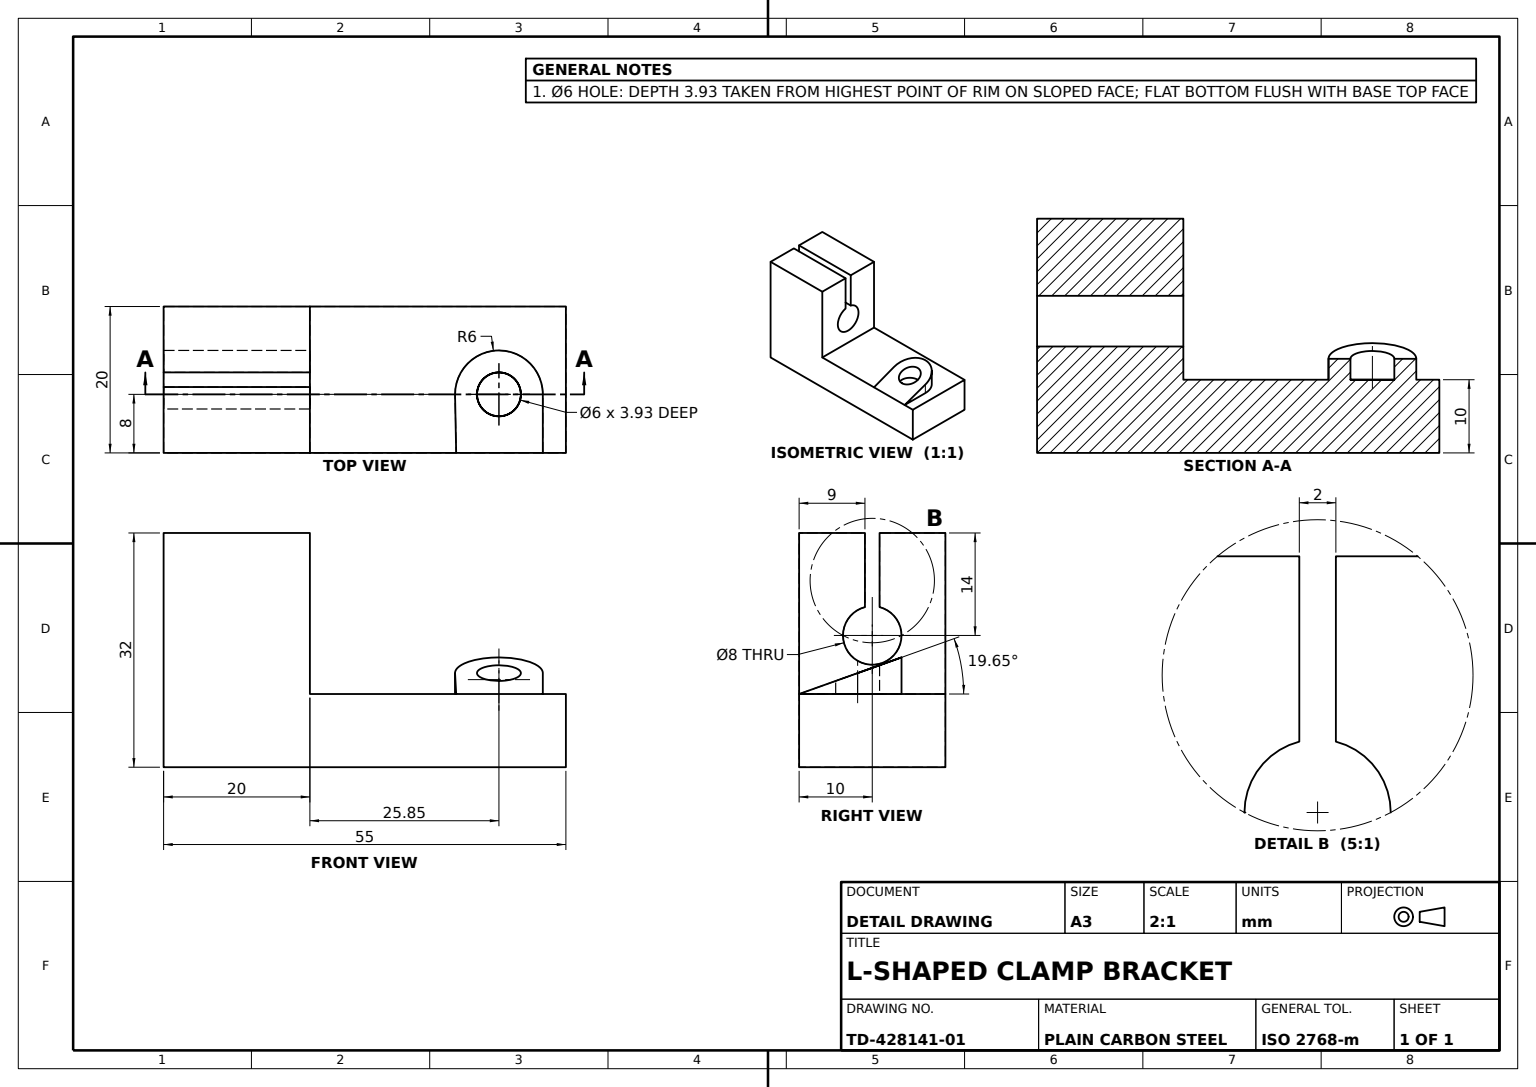
from build123d import *

# Parameters (mm, degrees)
L_BRACKET_BODY_DEPTH = 20
CLAMP_BORE_SKETCH_R  = 4
CLAMP_BORE_DEPTH     = 52.46843693
CLAMP_SLIT_DEPTH     = 52.46843693
CLEVIS_LUG_SKETCH_R  = 3
CLEVIS_LUG_DEPTH     = 5
LUG_PIN_HOLE_DEPTH   = 12


with BuildPart() as part:
    # Bracket Profile Sketch → L-Bracket Body (new body)
    with BuildSketch(Plane.XY):
        Polygon((0, 0), (55, 0), (55, 10), (20, 10), (20, 32), (0, 32), align=None)
    extrude(amount=L_BRACKET_BODY_DEPTH)

    # Clamp Bore Sketch → Clamp Bore (cut, through all)
    with BuildSketch(Plane(origin=(20, 0, 0), x_dir=(0, 0, -1), z_dir=(1, 0, 0))):
        with Locations((-10, 18)):
            Circle(CLAMP_BORE_SKETCH_R)
    extrude(amount=-CLAMP_BORE_DEPTH, mode=Mode.SUBTRACT)

    # Clamp Slit Sketch → Clamp Slit (cut, through all)
    with BuildSketch(Plane(origin=(20, 0, 0), x_dir=(0, 0, -1), z_dir=(1, 0, 0))):
        with BuildLine():
            ThreePointArc((-11, 21.872983346), (-10, 22), (-9, 21.872983346))
            Line((-9, 21.872983346), (-9, 32))
            Line((-9, 32), (-11, 32))
            Line((-11, 32), (-11, 21.872983346))
        make_face()
    extrude(amount=-CLAMP_SLIT_DEPTH, mode=Mode.SUBTRACT)

    # Clevis Lug Sketch → Clevis Lug (add)
    with BuildSketch(Plane(origin=(0, 10, 0), x_dir=(1, 0, 0), z_dir=(0, 1, 0))):
        with BuildLine():
            Line((39.847164106, -12.116295981), (40, -20))
            Line((40, -20), (51.846036937, -20))
            Line((51.846036937, -20), (51.846036937, -12))
            ThreePointArc((51.846036937, -12), (45.787886215, -6.000281799), (39.847164106, -12.116295981))
        make_face()
        with Locations(Location((45.846036937, -12, 0), (0, 0, 270))):
            Circle(CLEVIS_LUG_SKETCH_R, mode=Mode.SUBTRACT)
    extrude(amount=CLEVIS_LUG_DEPTH)

    # Lug Pin Hole Sketch → Lug Pin Hole (cut)
    with BuildSketch(Plane(origin=(51.846036937, 0, 0), x_dir=(0, 0, -1), z_dir=(1, 0, 0))):
        Polygon((-20, 15), (-20, 10), (-6, 15), align=None)
    extrude(amount=-LUG_PIN_HOLE_DEPTH, mode=Mode.SUBTRACT)


solid = part.part
